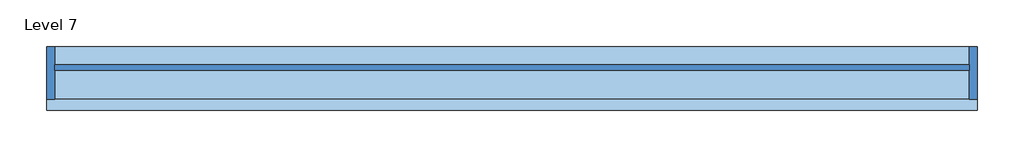
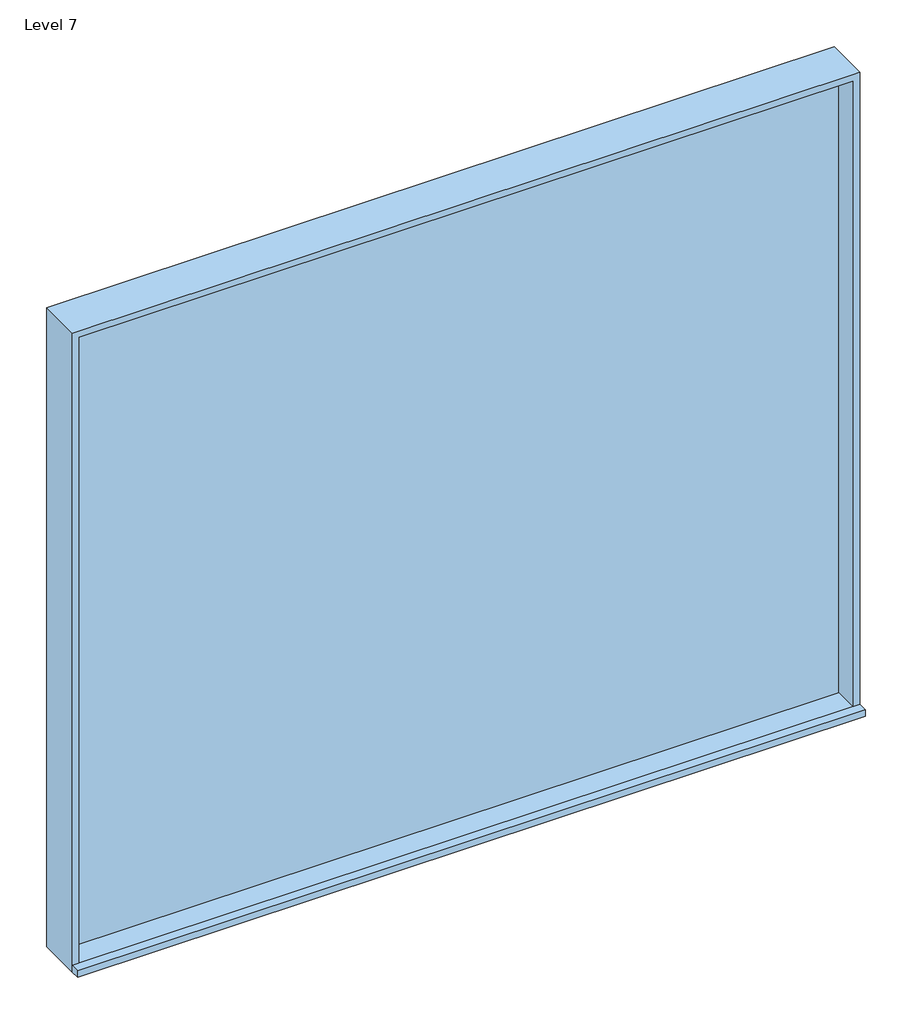
# One storey: 1 window.
"""IFC4 building model written with IfcOpenShell, lengths in millimetres."""

from ifc_helpers import new_model, si_unit, origin, place, context, project, spatial, transform, mapped, element, save
from components import window_88b07bfa

model = new_model("IFC4")

# Units and contexts
model_context = context("Model", 3, world=origin())
ifc_project = project(units=[si_unit("LENGTHUNIT", "METRE", prefix="MILLI")], contexts=[model_context])

# Site, building, storey
site = spatial("IfcSite", under=ifc_project)
building = spatial("IfcBuilding", under=site)
storey = spatial("IfcBuildingStorey", under=building, Name="Level 7", Elevation=18288.0)

# Window
placement = place(None, origin())
window_shape = window_88b07bfa(model_context)
element("IfcWindow", 1, ObjectType="Instance - Fixed : 24\" x 48\"", at=placement, inside=storey, context=model_context, shape_type="MappedRepresentation", body=[
    mapped(window_shape, transform((-10747.8874719, -885.9632813, 17312.2483945), x_axis=(-1.0, 0.0, 0.0), y_axis=(0.0, -1.0, 0.0), z_axis=(0.0, 0.0, 1.0))),
])

save(model, "model.ifc")

# Revit data of these elements
# Type "Instance - Fixed : 24\" x 48\""
#   Type Mark = "10"
#   Construction Type Id = "GSP4R"
#   Assembly Code = "B2020100"
#   Analytic Construction = "1/8 in Pilkington single glazing"
#   Visual Light Transmittance = 0.9
#   Thermal Resistance (R) = 0.8466 (h·ft²·°F)/BTU
#   Solar Heat Gain Coefficient = 0.86
#   Heat Transfer Coefficient (U) = 1.1812 BTU/(h·ft²·°F)
#   Height [instance default] = 4' - 0"
#   Default Sill Height = 3' - 0"
#   Width [instance default] = 2' - 0"
#   Window Inset = 0' - 2"
#   Define Thermal Properties by = 1
#   Glass Pane Material = Glass
#   Sash Material = Iron, Ductile
#   Wall Closure = (empty or 0)
# Element 1 (IfcWindow, "Instance - Fixed : 24\" x 48\"")
#   Mark = "6"
#   Width = 7' - 0"
#   Height = 6' - 0"
#   Phase Created = New Construction
#   Materials on its faces: "Iron, Ductile", "Glass"
# Materials
#   "Glass": class "Glass", colour RGB 0 128 192, transparency 0.75, Description = "Soda Lime Glass", Cost = 0
#   "Iron, Ductile": class "Metal", colour RGB 0 0 0, transparency 0, Description = "Ductile cast iron", Cost = 0
